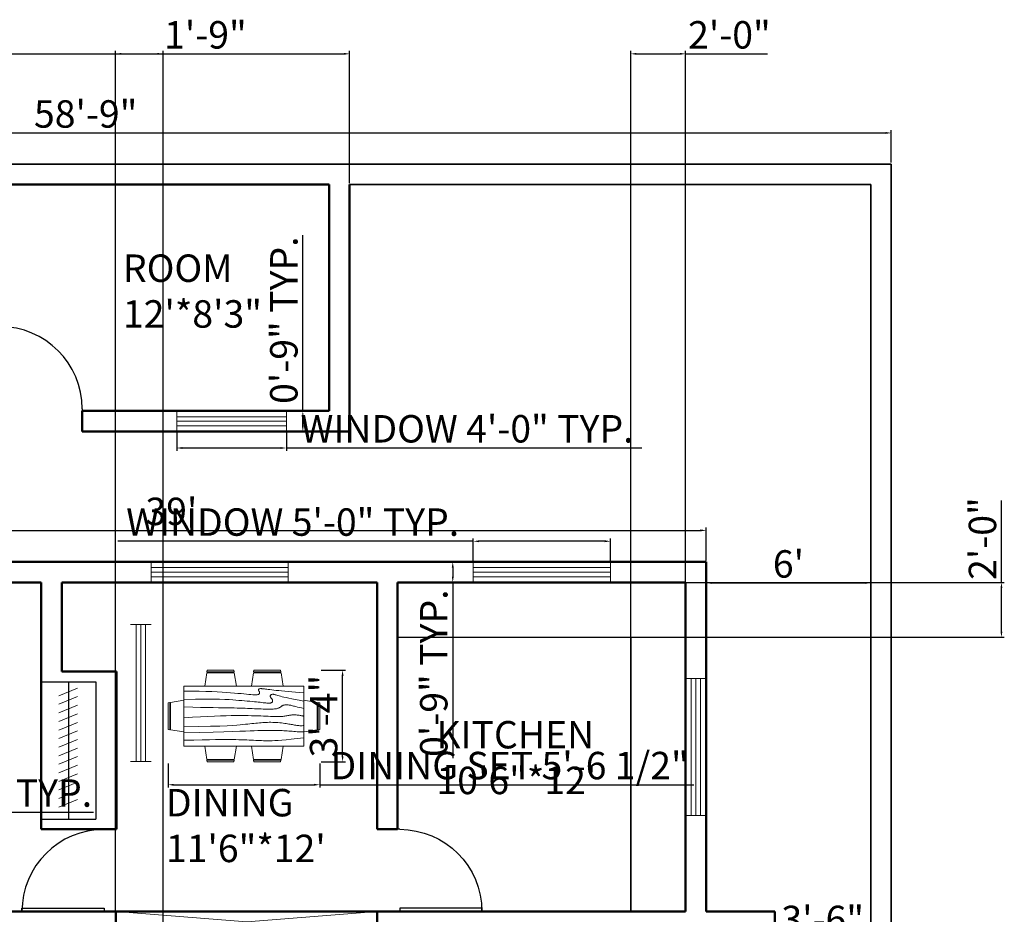
# Model space of a CAD drawing. Units: inches. Extents: x 6286 to 7213, y 5725 to 6776.
# Tile 5 of 5: x 6683 to 7113, y 6385 to 6776. Entities that reach past the tile are written whole.
import ezdxf

# ---------------------------------------------------------------- set-up
doc = ezdxf.new("R2010")
doc.units = ezdxf.units.IN
for name, color, linetype, lineweight in [('A-ANNO-DIMS', 2, 'Continuous', 18), ('A-AREA-IDEN', 7, 'Continuous', 25), ('A-DOOR', 3, 'Continuous', 25), ('A-FLOR-CASE', 8, 'Continuous', 25), ('A-FLOR-CASE-PATT', 252, 'Continuous', 13), ('A-FURN', 8, 'Continuous', 18), ('A-GLAZ', 4, 'Continuous', 18), ('A-WALL', 7, 'Continuous', 50), ('A-WALL-OPEN', 7, 'Continuous', 18), ('C-PROP', 7, 'Continuous', 35)]:
    doc.layers.add(name, color=color, linetype=linetype, lineweight=lineweight)
doc.styles.get("Standard").update_dxf_attribs({"font": 'arial.ttf'})
doc.dimstyles.new('ISO-25', dxfattribs={"dimtxt": 12, "dimasz": 2.5, "dimexe": 1.25, "dimexo": 0.625, "dimtad": 1, "dimdec": 1, "dimlunit": 4, "dimtxsty": 'Standard', "dimcen": 2.5, "dimadec": 0, "dimazin": 0, "dimtfac": 1, "dimtdec": 1, "dimtmove": 0, "dimatfit": 3, "dimfxl": 1, "dimarcsym": 0})

# ---------------------------------------------------------------- blocks, each defined once
blk = doc.blocks.new('*U2')
for p, q in [((0, 0), (0, -6)), ((40, 0), (40, -6))]:
    blk.add_line(p, q)
blk.add_lwpolyline([(0, 0), (0, 40), (1.75, 40), (1.75, 0)], close=True)
blk.add_arc((0, 0), 40, 0, 90)
blk = doc.blocks.new('*D3')
at = {"layer": 'A-ANNO-DIMS', "color": 0, "lineweight": -2, "transparency": 16777216}
for p, q in [((6358.92, 6713.89), (6358.92, 6728.11)), ((6361.42, 6726.86), (7061.42, 6726.86)), ((7063.92, 6713.89), (7063.92, 6728.11))]:
    blk.add_line(p, q, dxfattribs=at)
at = {"layer": 'A-ANNO-DIMS', "color": 0, "lineweight": 100, "transparency": 16777216}
for points in [[(6361.42, 6727.28), (6361.42, 6726.44), (6358.92, 6726.86)], [(7061.42, 6727.28), (7061.42, 6726.44), (7063.92, 6726.86)]]:
    blk.add_solid(points, dxfattribs=at)
at = {"layer": 'Defpoints', "color": 0, "lineweight": 100, "transparency": 16777216}
for p in [(7063.92, 6726.86), (6358.92, 6713.26), (7063.92, 6713.26)]:
    blk.add_point(p, dxfattribs=at)
at = {"layer": 'A-ANNO-DIMS', "color": 0, "transparency": 16777216, "insert": (6711.42, 6733.61), "char_height": 12, "attachment_point": 5}
blk.add_mtext('58\'-9"', dxfattribs=at)
blk = doc.blocks.new('*D5')
at = {"layer": 'A-ANNO-DIMS', "color": 0, "lineweight": -2, "transparency": 16777216}
for p, q in [((6514.92, 6539.89), (6514.92, 6554.27)), ((6517.42, 6553.02), (6980.42, 6553.02)), ((6982.92, 6539.89), (6982.92, 6554.27))]:
    blk.add_line(p, q, dxfattribs=at)
at = {"layer": 'A-ANNO-DIMS', "color": 0, "lineweight": 100, "transparency": 16777216}
for points in [[(6517.42, 6553.44), (6517.42, 6552.6), (6514.92, 6553.02)], [(6980.42, 6553.44), (6980.42, 6552.6), (6982.92, 6553.02)]]:
    blk.add_solid(points, dxfattribs=at)
at = {"layer": 'Defpoints', "color": 0, "lineweight": 100, "transparency": 16777216}
for p in [(6982.92, 6553.02), (6514.92, 6539.26), (6982.92, 6539.26)]:
    blk.add_point(p, dxfattribs=at)
at = {"layer": 'A-ANNO-DIMS', "color": 0, "transparency": 16777216, "insert": (6748.92, 6559.78), "char_height": 12, "attachment_point": 5}
blk.add_mtext("39'", dxfattribs=at)
blk = doc.blocks.new('Dining Set - 36 x 72 in.')
for p, q in [((-22.2343, 26.00059), (-23.4847, 17.99762)), ((-22.2304, 26), (-5.7608, 26)), ((-22, 27.5), (-22.1562, 26.50042)), ((-5.8416, 26.5), (-22.1534, 26.5)), ((-22, 27.5), (-6, 27.5)), ((-5.8437, 26.49966), (-6, 27.5)), ((-4.5152, 17.99762), (-5.7655, 25.99926)), ((5.7657, 26.00059), (4.5153, 17.99762)), ((5.7696, 26), (22.2392, 26)), ((6, 27.5), (5.8438, 26.50042)), ((22.1584, 26.5), (5.8466, 26.5)), ((6, 27.5), (22, 27.5)), ((22.1563, 26.49966), (22, 27.5)), ((23.4848, 17.99762), (22.2345, 25.99926)), ((36, 18), (-36, 18)), ((-36, 18), (-36, -18)), ((36, -18), (36, 18)), ((-45.5, 8), (-44.5004, 8.15617)), ((-45.5, 8), (-45.5, -8)), ((-44.5, -8.15843), (-44.5, 8.15338)), ((-44.0006, 8.23428), (-35.9976, 9.48474)), ((-44, 8.23041), (-44, -8.23915)), ((44.0006, 8.23428), (35.9976, 9.48474)), ((44, 8.23041), (44, -8.23915)), ((44.5, -8.15843), (44.5, 8.15338)), ((45.5, 8), (44.5005, 8.15617)), ((45.5, 8), (45.5, -8)), ((-44.4997, -8.15631), (-45.5, -8)), ((-35.9976, -9.48476), (-43.9993, -8.2345)), ((35.9976, -9.48476), (43.9993, -8.2345)), ((44.4997, -8.15631), (45.5, -8)), ((-36, -18), (36, -18)), ((-22.2343, -26.0006), (-23.4847, -17.99762)), ((-4.5152, -17.99762), (-5.7655, -25.99928)), ((5.7657, -26.0006), (4.5153, -17.99762)), ((23.4848, -17.99762), (22.2345, -25.99928)), ((-22.2304, -26), (-5.7608, -26)), ((-22, -27.5), (-22.1562, -26.50044)), ((-5.8416, -26.5), (-22.1534, -26.5)), ((-22, -27.5), (-6, -27.5)), ((-5.8437, -26.49967), (-6, -27.5)), ((5.7696, -26), (22.2392, -26)), ((6, -27.5), (5.8438, -26.50044)), ((22.1584, -26.5), (5.8466, -26.5)), ((6, -27.5), (22, -27.5)), ((22.1563, -26.49967), (22, -27.5))]:
    blk.add_line(p, q)
for points in [[(-36, 15), (-31.1772, 14.97754), (-26.8079, 14.91406), (-22.8538, 14.81543), (-19.276, 14.6875), (-16.0362, 14.53613), (-13.0957, 14.36718), (-10.4159, 14.18652), (-7.9583, 14), (-5.6904, 13.81315), (-3.6035, 13.63021), (-1.6954, 13.45508), (0.0365, 13.29166), (1.5945, 13.14388), (2.9811, 13.01562), (4.1988, 12.9108), (5.25, 12.83333), (6.1393, 12.78613), (6.8802, 12.76823), (7.4883, 12.77767), (7.9792, 12.8125), (8.3685, 12.87077), (8.6719, 12.95052), (8.9049, 13.0498), (9.0833, 13.16666), (9.2205, 13.29899), (9.3216, 13.44401), (9.3895, 13.59879), (9.4271, 13.76041), (9.4373, 13.92594), (9.4232, 14.09245), (9.3875, 14.257), (9.3333, 14.41666), (9.2638, 14.56917), (9.1836, 14.71484), (9.0975, 14.85465), (9.0104, 14.98958), (8.9272, 15.1206), (8.8529, 15.2487), (8.7922, 15.37483), (8.75, 15.5), (8.7305, 15.62467), (8.7344, 15.74739), (8.7617, 15.86621), (8.8125, 15.97916), (8.8867, 16.08431), (8.9844, 16.17968), (9.1055, 16.26334), (9.25, 16.33333), (9.4189, 16.38802), (9.6172, 16.42708), (9.8506, 16.45052), (10.125, 16.45833), (10.4463, 16.45052), (10.8203, 16.42708), (11.2529, 16.38802), (11.75, 16.33333), (12.3184, 16.26318), (12.9694, 16.17838), (13.7151, 16.07991), (14.5677, 15.96875), (15.5395, 15.84586), (16.6426, 15.71224), (17.8893, 15.56884), (19.2917, 15.41666), (20.859, 15.25667), (22.5879, 15.08984), (24.4721, 14.91715), (26.5052, 14.73958), (28.6809, 14.5581), (30.9929, 14.3737), (33.4347, 14.18733), (36, 14)], [(-36, 10), (-28.9766, 10.14274), (-23.1725, 10.20442), (-18.4241, 10.19775), (-14.5677, 10.13541), (-11.4399, 10.03011), (-8.877, 9.89453), (-6.7154, 9.74137), (-4.7917, 9.58333), (-2.9698, 9.43082), (-1.2246, 9.28515), (0.4415, 9.14534), (2.026, 9.01041), (3.5266, 8.87939), (4.9408, 8.7513), (6.266, 8.62516), (7.5, 8.5), (8.6411, 8.37549), (9.6914, 8.2539), (10.6538, 8.13818), (11.5312, 8.03125), (12.3267, 7.93603), (13.043, 7.85547), (13.6831, 7.79248), (14.25, 7.75), (14.7471, 7.7303), (15.1797, 7.73307), (15.5537, 7.75732), (15.875, 7.80208), (16.1494, 7.86637), (16.3828, 7.94922), (16.5811, 8.04964), (16.75, 8.16666), (16.8944, 8.29915), (17.0143, 8.44531), (17.1089, 8.60319), (17.1771, 8.77083), (17.218, 8.94629), (17.2305, 9.1276), (17.2137, 9.31282), (17.1667, 9.5), (17.0895, 9.6875), (16.987, 9.875), (16.8649, 10.0625), (16.7292, 10.25), (16.5856, 10.4375), (16.4401, 10.625), (16.2985, 10.8125), (16.1667, 11), (16.05, 11.18733), (15.9518, 11.3737), (15.8752, 11.5581), (15.8229, 11.73958), (15.798, 11.91715), (15.8034, 12.08984), (15.842, 12.25667), (15.9167, 12.41666), (16.0295, 12.56836), (16.1784, 12.70833), (16.3605, 12.83268), (16.5729, 12.9375), (16.8127, 13.01888), (17.0768, 13.07291), (17.3625, 13.0957), (17.6667, 13.08333), (17.9894, 13.03312), (18.3418, 12.94726), (18.7382, 12.82918), (19.1927, 12.68229), (19.7195, 12.51001), (20.3327, 12.31575), (21.0465, 12.10294), (21.875, 11.875), (22.8357, 11.63354), (23.959, 11.37304), (25.2786, 11.08618), (26.8282, 10.76562), (28.6414, 10.40405), (30.752, 9.99414), (33.1936, 9.52856), (36, 9)], [(-36, 5.5), (-30.7157, 5.3348), (-26.069, 5.20963), (-21.9946, 5.11767), (-18.4271, 5.05208), (-15.3009, 5.00602), (-12.5508, 4.97265), (-10.1112, 4.94515), (-7.9167, 4.91666), (-5.909, 4.88167), (-4.0586, 4.83984), (-2.3429, 4.79215), (-0.7396, 4.73958), (0.7739, 4.6831), (2.22, 4.6237), (3.6213, 4.56233), (5, 4.5), (6.373, 4.43782), (7.7344, 4.3776), (9.0723, 4.32129), (10.375, 4.27083), (11.6309, 4.22819), (12.8281, 4.19531), (13.9551, 4.17415), (15, 4.16666), (15.954, 4.17448), (16.819, 4.19791), (17.6001, 4.23698), (18.3021, 4.29166), (18.9299, 4.36198), (19.4883, 4.44791), (19.9823, 4.54948), (20.4167, 4.66666), (20.7969, 4.79899), (21.1302, 4.94401), (21.4245, 5.09879), (21.6875, 5.26041), (21.9271, 5.42594), (22.1511, 5.59245), (22.3672, 5.757), (22.5834, 5.91666), (22.8065, 6.06868), (23.0404, 6.21093), (23.2879, 6.34147), (23.5521, 6.45833), (23.8358, 6.55957), (24.142, 6.64323), (24.4735, 6.70735), (24.8334, 6.75), (25.2235, 6.76969), (25.642, 6.76692), (26.0858, 6.74267), (26.5521, 6.69791), (27.0379, 6.63362), (27.5404, 6.55078), (28.0565, 6.45036), (28.5834, 6.33333), (29.1242, 6.19987), (29.7071, 6.04687), (30.3661, 5.87044), (31.1354, 5.66666), (32.0493, 5.43164), (33.142, 5.16146), (34.4475, 4.85221), (36, 4.5)], [(-36, -1), (-30.7915, -0.6591), (-26.0195, -0.38216), (-21.6519, -0.16284), (-17.6563, 0.00521), (-14.0005, 0.12833), (-10.6523, 0.21289), (-7.5796, 0.26522), (-4.75, 0.29166), (-2.134, 0.29793), (0.2878, 0.28711), (2.5317, 0.26163), (4.6146, 0.22396), (6.5529, 0.17651), (8.3633, 0.12174), (10.0623, 0.06209), (11.6667, 0), (13.1899, -0.06201), (14.6341, -0.1211), (15.9982, -0.17432), (17.2813, -0.21875), (18.4823, -0.25147), (19.6003, -0.26953), (20.6343, -0.27002), (21.5834, -0.25), (22.4481, -0.20768), (23.2357, -0.14584), (23.9549, -0.06836), (24.6146, 0.02083), (25.2235, 0.11784), (25.7904, 0.21875), (26.3241, 0.31966), (26.8334, 0.41666), (27.3265, 0.50618), (27.8099, 0.58593), (28.2894, 0.65397), (28.7709, 0.70833), (29.2601, 0.74707), (29.763, 0.76823), (30.2855, 0.76985), (30.8334, 0.75), (31.4088, 0.70784), (31.9994, 0.64713), (32.589, 0.57275), (33.1615, 0.48958), (33.7008, 0.4025), (34.1908, 0.3164), (34.6153, 0.23616), (34.9584, 0.16666), (35.2099, 0.11165), (35.3848, 0.07031), (35.504, 0.04069), (35.5886, 0.02083), (35.6594, 0.00879), (35.7377, 0.0026), (35.8442, 0.00032), (36, 0)], [(-36, -6.5), (-27.1843, -6.31267), (-20.084, -6.1263), (-14.469, -5.9419), (-10.1094, -5.76042), (-6.7752, -5.58285), (-4.2363, -5.41016), (-2.2629, -5.24333), (-0.625, -5.08334), (0.8708, -4.93099), (2.2715, -4.78646), (3.5872, -4.64974), (4.8281, -4.52084), (6.0046, -4.39974), (7.127, -4.28646), (8.2053, -4.18099), (9.25, -4.08334), (10.2705, -3.99382), (11.2734, -3.91407), (12.2647, -3.84603), (13.25, -3.79167), (14.2354, -3.75293), (15.2266, -3.73177), (16.2295, -3.73015), (17.25, -3.75), (18.2912, -3.79248), (19.3451, -3.85547), (20.4009, -3.93604), (21.4479, -4.03125), (22.4754, -4.13819), (23.4727, -4.25391), (24.4289, -4.37549), (25.3334, -4.5), (26.1785, -4.62492), (26.9694, -4.74935), (27.7145, -4.87281), (28.4219, -4.99479), (29.1, -5.11483), (29.7572, -5.23242), (30.4016, -5.34709), (31.0417, -5.45834), (31.6837, -5.56437), (32.3262, -5.65821), (32.9658, -5.73153), (33.599, -5.77604), (34.2224, -5.78345), (34.8327, -5.74545), (35.4264, -5.65373), (36, -5.5)], [(-36, -10), (-26.4022, -9.81299), (-18.4675, -9.62891), (-11.9839, -9.45069), (-6.7396, -9.28125), (-2.5226, -9.12354), (0.8789, -8.98047), (3.6769, -8.85498), (6.0833, -8.75), (8.2767, -8.66765), (10.3021, -8.60677), (12.1712, -8.56543), (13.8958, -8.54167), (15.4876, -8.53353), (16.9583, -8.53907), (18.3197, -8.55632), (19.5834, -8.58334), (20.7616, -8.61841), (21.8685, -8.66081), (22.9188, -8.71004), (23.9271, -8.76563), (24.9081, -8.82707), (25.8763, -8.89388), (26.8465, -8.96558), (27.8334, -9.04167), (28.8474, -9.12118), (29.8828, -9.20117), (30.93, -9.27824), (31.9792, -9.34896), (33.0205, -9.40991), (34.0443, -9.45768), (35.0407, -9.48885), (36, -9.5)], [(-36, -14.5), (-30.0881, -14.33513), (-25.0332, -14.21224), (-20.7312, -14.12647), (-17.0781, -14.07292), (-13.97, -14.04671), (-11.3027, -14.04297), (-8.9724, -14.05681), (-6.875, -14.08334), (-4.9224, -14.11833), (-3.0905, -14.16016), (-1.3709, -14.20785), (0.2448, -14.26042), (1.7647, -14.3169), (3.1973, -14.3763), (4.5507, -14.43767), (5.8333, -14.5), (7.0554, -14.5621), (8.235, -14.62175), (9.3922, -14.67652), (10.5469, -14.72396), (11.7192, -14.76164), (12.929, -14.78711), (14.1965, -14.79794), (15.5417, -14.79167), (16.9933, -14.76424), (18.6152, -14.70508), (20.4804, -14.60197), (22.6615, -14.44271), (25.2312, -14.21509), (28.2624, -13.9069), (31.8277, -13.50594), (36, -13)]]:
    blk.add_lwpolyline(points)
blk = doc.blocks.new('*D23')
at = {"layer": 'A-ANNO-DIMS', "color": 0, "lineweight": -2, "transparency": 16777216}
for p, q in [((6982.92, 6538.64), (6982.92, 6528.79)), ((7054.92, 6538.64), (7054.92, 6528.79)), ((6985.42, 6530.04), (7052.42, 6530.04))]:
    blk.add_line(p, q, dxfattribs=at)
at = {"layer": 'A-ANNO-DIMS', "color": 0, "lineweight": 100, "transparency": 16777216}
for points in [[(6985.42, 6530.45), (6985.42, 6529.62), (6982.92, 6530.04)], [(7052.42, 6530.45), (7052.42, 6529.62), (7054.92, 6530.04)]]:
    blk.add_solid(points, dxfattribs=at)
at = {"layer": 'Defpoints', "color": 0, "lineweight": 100, "transparency": 16777216}
for p in [(6982.92, 6539.26), (7054.92, 6539.26), (7054.92, 6530.04)]:
    blk.add_point(p, dxfattribs=at)
at = {"layer": 'A-ANNO-DIMS', "color": 0, "transparency": 16777216, "insert": (7018.92, 6536.79), "char_height": 12, "attachment_point": 5}
blk.add_mtext("6'", dxfattribs=at)
blk = doc.blocks.new('*D24')
at = {"layer": 'A-ANNO-DIMS', "color": 0, "lineweight": -2, "transparency": 16777216}
for p, q in [((7012.92, 6385.64), (7012.92, 6373.28)), ((7054.92, 6385.64), (7054.92, 6373.28)), ((7015.42, 6374.53), (7052.42, 6374.53))]:
    blk.add_line(p, q, dxfattribs=at)
at = {"layer": 'A-ANNO-DIMS', "color": 0, "lineweight": 100, "transparency": 16777216}
for points in [[(7015.42, 6374.95), (7015.42, 6374.12), (7012.92, 6374.53)], [(7052.42, 6374.95), (7052.42, 6374.12), (7054.92, 6374.53)]]:
    blk.add_solid(points, dxfattribs=at)
at = {"layer": 'Defpoints', "color": 0, "lineweight": 100, "transparency": 16777216}
for p in [(7012.92, 6386.26), (7054.92, 6386.26), (7054.92, 6374.53)]:
    blk.add_point(p, dxfattribs=at)
at = {"layer": 'A-ANNO-DIMS', "color": 0, "transparency": 16777216, "insert": (7033.92, 6381.29), "char_height": 12, "attachment_point": 5}
blk.add_mtext('3\'-6"', dxfattribs=at)
blk = doc.blocks.new('WIN-48IN')
for p, q in [((0, 9), (0, 0)), ((48, 0), (48, 9)), ((0, 6.5), (48, 6.5)), ((0, 4.5), (48, 4.5)), ((0, 2.5), (48, 2.5))]:
    blk.add_line(p, q)
blk = doc.blocks.new('WIN-60IN')
for p, q in [((0, 9), (0, 0)), ((60, 0), (60, 9)), ((60, 6.5), (0, 6.5)), ((60, 4.5), (0, 4.5)), ((60, 2.5), (0, 2.5))]:
    blk.add_line(p, q)
blk = doc.blocks.new('*D35')
at = {"layer": 'A-ANNO-DIMS', "color": 0, "lineweight": -2, "transparency": 16777216}
for p, q in [((6881.04, 6539.89), (6881.04, 6549.51)), ((6941.04, 6539.89), (6941.04, 6549.51)), ((6881.04, 6548.26), (6725.44, 6548.26)), ((6938.54, 6548.26), (6883.54, 6548.26))]:
    blk.add_line(p, q, dxfattribs=at)
at = {"layer": 'A-ANNO-DIMS', "color": 0, "lineweight": 100, "transparency": 16777216}
for points in [[(6883.54, 6548.68), (6883.54, 6547.85), (6881.04, 6548.26)], [(6938.54, 6548.68), (6938.54, 6547.85), (6941.04, 6548.26)]]:
    blk.add_solid(points, dxfattribs=at)
at = {"layer": 'Defpoints', "color": 0, "lineweight": 100, "transparency": 16777216}
for p in [(6881.04, 6548.26), (6881.04, 6539.26), (6941.04, 6539.26)]:
    blk.add_point(p, dxfattribs=at)
at = {"layer": 'A-ANNO-DIMS', "color": 0, "transparency": 16777216, "insert": (6801.99, 6555.1), "char_height": 12, "attachment_point": 5}
blk.add_mtext('WINDOW 5\'-0" TYP.', dxfattribs=at)
blk = doc.blocks.new('*D36')
at = {"layer": 'A-ANNO-DIMS', "color": 0, "lineweight": -2, "transparency": 16777216}
for p, q in [((6880.42, 6539.26), (6870.79, 6539.26)), ((6872.04, 6536.76), (6872.04, 6532.76)), ((6880.42, 6530.26), (6870.79, 6530.26)), ((6872.04, 6530.26), (6872.04, 6453.37))]:
    blk.add_line(p, q, dxfattribs=at)
at = {"layer": 'A-ANNO-DIMS', "color": 0, "lineweight": 100, "transparency": 16777216}
for points in [[(6871.63, 6536.76), (6872.46, 6536.76), (6872.04, 6539.26)], [(6871.63, 6532.76), (6872.46, 6532.76), (6872.04, 6530.26)]]:
    blk.add_solid(points, dxfattribs=at)
at = {"layer": 'Defpoints', "color": 0, "lineweight": 100, "transparency": 16777216}
for p in [(6881.04, 6539.26), (6872.04, 6530.26), (6881.04, 6530.26)]:
    blk.add_point(p, dxfattribs=at)
at = {"layer": 'A-ANNO-DIMS', "color": 0, "transparency": 16777216, "insert": (6865.29, 6490.57), "char_height": 12, "attachment_point": 5, "rotation": 90}
blk.add_mtext('0\'-9" TYP.', dxfattribs=at)
blk = doc.blocks.new('*D37')
at = {"layer": 'A-ANNO-DIMS', "color": 0, "lineweight": -2, "transparency": 16777216}
for p, q in [((6751.24, 6595.64), (6751.24, 6587.81)), ((6799.24, 6595.64), (6799.24, 6587.81)), ((6753.74, 6589.06), (6796.74, 6589.06)), ((6799.24, 6589.06), (6954.84, 6589.06))]:
    blk.add_line(p, q, dxfattribs=at)
at = {"layer": 'A-ANNO-DIMS', "color": 0, "lineweight": 100, "transparency": 16777216}
for points in [[(6753.74, 6589.48), (6753.74, 6588.65), (6751.24, 6589.06)], [(6796.74, 6589.48), (6796.74, 6588.65), (6799.24, 6589.06)]]:
    blk.add_solid(points, dxfattribs=at)
at = {"layer": 'Defpoints', "color": 0, "lineweight": 100, "transparency": 16777216}
for p in [(6751.24, 6596.26), (6799.24, 6596.26), (6799.24, 6589.06)]:
    blk.add_point(p, dxfattribs=at)
at = {"layer": 'A-ANNO-DIMS', "color": 0, "transparency": 16777216, "insert": (6878.29, 6595.9), "char_height": 12, "attachment_point": 5}
blk.add_mtext('WINDOW 4\'-0" TYP.', dxfattribs=at)
blk = doc.blocks.new('*D38')
at = {"layer": 'A-ANNO-DIMS', "color": 0, "lineweight": -2, "transparency": 16777216}
for p, q in [((6806.44, 6605.26), (6806.44, 6682.16)), ((6799.86, 6605.26), (6807.69, 6605.26)), ((6806.44, 6598.76), (6806.44, 6602.76)), ((6799.86, 6596.26), (6807.69, 6596.26))]:
    blk.add_line(p, q, dxfattribs=at)
at = {"layer": 'A-ANNO-DIMS', "color": 0, "lineweight": 100, "transparency": 16777216}
for points in [[(6806.02, 6602.76), (6806.85, 6602.76), (6806.44, 6605.26)], [(6806.02, 6598.76), (6806.85, 6598.76), (6806.44, 6596.26)]]:
    blk.add_solid(points, dxfattribs=at)
at = {"layer": 'Defpoints', "color": 0, "lineweight": 100, "transparency": 16777216}
for p in [(6799.24, 6605.26), (6806.44, 6605.26), (6799.24, 6596.26)]:
    blk.add_point(p, dxfattribs=at)
at = {"layer": 'A-ANNO-DIMS', "color": 0, "transparency": 16777216, "insert": (6799.68, 6644.96), "char_height": 12, "attachment_point": 5, "rotation": 90}
blk.add_mtext('0\'-9" TYP.', dxfattribs=at)
blk = doc.blocks.new('*D48')
at = {"layer": 'A-ANNO-DIMS', "color": 0, "lineweight": -2, "transparency": 16777216}
for p, q in [((6577.92, 6442.12), (6577.92, 6428.58)), ((6637.92, 6442.12), (6637.92, 6428.58)), ((6580.42, 6429.83), (6635.42, 6429.83)), ((6637.92, 6429.83), (6714.82, 6429.83))]:
    blk.add_line(p, q, dxfattribs=at)
at = {"layer": 'A-ANNO-DIMS', "color": 0, "lineweight": 100, "transparency": 16777216}
for points in [[(6580.42, 6430.25), (6580.42, 6429.42), (6577.92, 6429.83)], [(6635.42, 6430.25), (6635.42, 6429.42), (6637.92, 6429.83)]]:
    blk.add_solid(points, dxfattribs=at)
at = {"layer": 'Defpoints', "color": 0, "lineweight": 100, "transparency": 16777216}
for p in [(6577.92, 6442.75), (6637.92, 6442.75), (6637.92, 6429.83)]:
    blk.add_point(p, dxfattribs=at)
at = {"layer": 'A-ANNO-DIMS', "color": 0, "transparency": 16777216, "insert": (6677.62, 6436.59), "char_height": 12, "attachment_point": 5}
blk.add_mtext('5\'-0" TYP.', dxfattribs=at)
blk = doc.blocks.new('*D51')
at = {"layer": 'A-ANNO-DIMS', "color": 0, "lineweight": -2, "transparency": 16777216}
for p, q in [((6747.45, 6451.1), (6747.45, 6440.51)), ((6813.87, 6451.1), (6813.87, 6440.51)), ((6749.95, 6441.76), (6811.37, 6441.76)), ((6813.87, 6441.76), (6977.48, 6441.76))]:
    blk.add_line(p, q, dxfattribs=at)
at = {"layer": 'A-ANNO-DIMS', "color": 0, "lineweight": 100, "transparency": 16777216}
for points in [[(6749.95, 6442.17), (6749.95, 6441.34), (6747.45, 6441.76)], [(6811.37, 6442.17), (6811.37, 6441.34), (6813.87, 6441.76)]]:
    blk.add_solid(points, dxfattribs=at)
at = {"layer": 'Defpoints', "color": 0, "lineweight": 100, "transparency": 16777216}
for p in [(6747.45, 6451.72), (6813.87, 6451.72), (6813.87, 6441.76)]:
    blk.add_point(p, dxfattribs=at)
at = {"layer": 'A-ANNO-DIMS', "color": 0, "transparency": 16777216, "insert": (6896.92, 6448.59), "char_height": 12, "attachment_point": 5}
blk.add_mtext('DINING SET 5\'-6 1/2"', dxfattribs=at)
blk = doc.blocks.new('*D52')
at = {"layer": 'A-ANNO-DIMS', "color": 0, "lineweight": -2, "transparency": 16777216}
for p, q in [((6814.5, 6491.87), (6825.08, 6491.87)), ((6823.83, 6454.22), (6823.83, 6489.37)), ((6814.5, 6451.72), (6825.08, 6451.72))]:
    blk.add_line(p, q, dxfattribs=at)
at = {"layer": 'A-ANNO-DIMS', "color": 0, "lineweight": 100, "transparency": 16777216}
for points in [[(6823.42, 6489.37), (6824.25, 6489.37), (6823.83, 6491.87)], [(6823.42, 6454.22), (6824.25, 6454.22), (6823.83, 6451.72)]]:
    blk.add_solid(points, dxfattribs=at)
at = {"layer": 'Defpoints', "color": 0, "lineweight": 100, "transparency": 16777216}
for p in [(6813.87, 6491.87), (6823.83, 6491.87), (6813.87, 6451.72)]:
    blk.add_point(p, dxfattribs=at)
at = {"layer": 'A-ANNO-DIMS', "color": 0, "transparency": 16777216, "insert": (6817.08, 6471.79), "char_height": 12, "attachment_point": 5, "rotation": 90}
blk.add_mtext('3\'-4"', dxfattribs=at)
blk = doc.blocks.new('*D57')
at = {"layer": 'A-ANNO-DIMS', "color": 0, "lineweight": -2, "transparency": 16777216}
for p, q in [((6358.92, 6713.89), (6358.92, 6762.71)), ((6361.42, 6761.46), (6824.42, 6761.46)), ((6826.92, 6704.89), (6826.92, 6762.71))]:
    blk.add_line(p, q, dxfattribs=at)
at = {"layer": 'A-ANNO-DIMS', "color": 0, "lineweight": 100, "transparency": 16777216}
for points in [[(6361.42, 6761.88), (6361.42, 6761.05), (6358.92, 6761.46)], [(6824.42, 6761.88), (6824.42, 6761.05), (6826.92, 6761.46)]]:
    blk.add_solid(points, dxfattribs=at)
at = {"layer": 'Defpoints', "color": 0, "lineweight": 100, "transparency": 16777216}
for p in [(6826.92, 6761.46), (6358.92, 6713.26), (6826.92, 6704.26)]:
    blk.add_point(p, dxfattribs=at)
at = {"layer": 'A-ANNO-DIMS', "color": 0, "transparency": 16777216, "insert": (6592.92, 6768.22), "char_height": 12, "attachment_point": 5}
blk.add_mtext('39\'-0"', dxfattribs=at)
blk = doc.blocks.new('*D64')
at = {"layer": 'A-ANNO-DIMS', "color": 0, "lineweight": -2, "transparency": 16777216}
for p, q in [((6724.5, 6312.3), (6724.5, 6762.71)), ((6727, 6761.46), (6742.8, 6761.46)), ((6745.3, 6312.3), (6745.3, 6762.71)), ((6745.3, 6761.46), (6779.82, 6761.46))]:
    blk.add_line(p, q, dxfattribs=at)
at = {"layer": 'A-ANNO-DIMS', "color": 0, "lineweight": 100, "transparency": 16777216}
for points in [[(6727, 6761.88), (6727, 6761.05), (6724.5, 6761.46)], [(6742.8, 6761.88), (6742.8, 6761.05), (6745.3, 6761.46)]]:
    blk.add_solid(points, dxfattribs=at)
at = {"layer": 'Defpoints', "color": 0, "lineweight": 100, "transparency": 16777216}
for p in [(6745.3, 6761.46), (6724.5, 6311.67), (6745.3, 6311.67)]:
    blk.add_point(p, dxfattribs=at)
at = {"layer": 'A-ANNO-DIMS', "color": 0, "transparency": 16777216, "insert": (6763.81, 6768.22), "char_height": 12, "attachment_point": 5}
blk.add_mtext('1\'-9"', dxfattribs=at)
blk = doc.blocks.new('*D71')
at = {"layer": 'A-ANNO-DIMS', "color": 0, "lineweight": -2, "transparency": 16777216}
for p, q in [((7112.12, 6530.26), (7112.12, 6566.12)), ((6848.55, 6530.26), (7113.37, 6530.26)), ((7112.12, 6508.76), (7112.12, 6527.76)), ((6848.55, 6506.26), (7113.37, 6506.26))]:
    blk.add_line(p, q, dxfattribs=at)
at = {"layer": 'A-ANNO-DIMS', "color": 0, "lineweight": 100, "transparency": 16777216}
for points in [[(7111.71, 6527.76), (7112.54, 6527.76), (7112.12, 6530.26)], [(7111.71, 6508.76), (7112.54, 6508.76), (7112.12, 6506.26)]]:
    blk.add_solid(points, dxfattribs=at)
at = {"layer": 'Defpoints', "color": 0, "lineweight": 100, "transparency": 16777216}
for p in [(6847.92, 6530.26), (7112.12, 6530.26), (6847.92, 6506.26)]:
    blk.add_point(p, dxfattribs=at)
at = {"layer": 'A-ANNO-DIMS', "color": 0, "transparency": 16777216, "insert": (7105.37, 6549.44), "char_height": 12, "attachment_point": 5, "rotation": 90}
blk.add_mtext('2\'-0"', dxfattribs=at)
blk = doc.blocks.new('*D72')
at = {"layer": 'A-ANNO-DIMS', "color": 0, "lineweight": -2, "transparency": 16777216}
for p, q in [((6949.92, 6386.89), (6949.92, 6762.71)), ((6952.42, 6761.46), (6971.42, 6761.46)), ((6973.92, 6386.89), (6973.92, 6762.71)), ((6973.92, 6761.46), (7009.78, 6761.46))]:
    blk.add_line(p, q, dxfattribs=at)
at = {"layer": 'A-ANNO-DIMS', "color": 0, "lineweight": 100, "transparency": 16777216}
for points in [[(6952.42, 6761.88), (6952.42, 6761.05), (6949.92, 6761.46)], [(6971.42, 6761.88), (6971.42, 6761.05), (6973.92, 6761.46)]]:
    blk.add_solid(points, dxfattribs=at)
at = {"layer": 'Defpoints', "color": 0, "lineweight": 100, "transparency": 16777216}
for p in [(6973.92, 6761.46), (6949.92, 6386.26), (6973.92, 6386.26)]:
    blk.add_point(p, dxfattribs=at)
at = {"layer": 'A-ANNO-DIMS', "color": 0, "transparency": 16777216, "insert": (6993.1, 6768.22), "char_height": 12, "attachment_point": 5}
blk.add_mtext('2\'-0"', dxfattribs=at)

msp = doc.modelspace()

# ---------------------------------------------------------------- hatches: boundary and pattern name
at = {"layer": 'A-FLOR-CASE-PATT'}
h = msp.add_hatch(dxfattribs=at)
h.set_pattern_fill('ANSI31', color=256, scale=1.091306, angle=-22.636, style=0)
h.paths.add_polyline_path([(6699.63, 6428.66), (6707.78, 6432.02), (6707.78, 6484.47), (6699.63, 6481.12)])

# ---------------------------------------------------------------- linework, layer by layer
at = {"layer": 'A-FLOR-CASE'}
for p, q in [((6847.92, 6506.26), (6949.92, 6506.26)), ((6949.92, 6506.26), (6949.92, 6386.26)), ((6691.92, 6486.76), (6715.92, 6486.76)), ((6703.92, 6486.76), (6703.92, 6426.76)), ((6715.92, 6486.76), (6715.92, 6426.76)), ((6691.92, 6426.76), (6715.92, 6426.76))]:
    msp.add_line(p, q, dxfattribs=at)
at = {"layer": 'A-WALL'}
for p, q in [((6673.92, 6704.26), (6817.92, 6704.26)), ((6817.92, 6704.26), (6817.92, 6605.26)), ((6826.92, 6704.26), (6826.92, 6596.26)), ((6709.92, 6605.26), (6817.92, 6605.26)), ((6709.92, 6605.26), (6709.92, 6596.26)), ((6709.92, 6596.26), (6826.92, 6596.26)), ((6514.92, 6539.26), (6982.92, 6539.26)), ((6982.92, 6539.26), (6982.92, 6386.26)), ((6523.92, 6530.26), (6691.92, 6530.26)), ((6691.92, 6530.26), (6691.92, 6422.26)), ((6700.92, 6530.26), (6700.92, 6491.26)), ((6700.92, 6530.26), (6838.92, 6530.26)), ((6838.92, 6530.26), (6838.92, 6422.26)), ((6847.92, 6530.26), (6847.92, 6422.26)), ((6847.92, 6530.26), (6973.92, 6530.26)), ((6973.92, 6530.26), (6973.92, 6386.26)), ((6700.92, 6491.26), (6724.92, 6491.26)), ((6724.92, 6491.26), (6724.92, 6422.26)), ((6691.92, 6422.26), (6724.92, 6422.26)), ((6838.92, 6422.26), (6847.92, 6422.26)), ((6838.92, 6386.26), (6523.92, 6386.26)), ((6838.92, 6386.26), (6838.92, 6117.76)), ((6838.92, 6386.26), (6847.92, 6386.26)), ((6847.92, 6386.26), (6973.92, 6386.26)), ((6982.92, 6386.26), (7012.92, 6386.26)), ((7012.92, 6386.26), (7012.92, 6230.26))]:
    msp.add_line(p, q, dxfattribs=at)
at = {"layer": 'A-WALL-OPEN'}
for p, q in [((6724.92, 6386.26), (6724.92, 6377.26)), ((6724.92, 6386.26), (6838.92, 6377.26)), ((6838.92, 6386.26), (6724.92, 6377.26))]:
    msp.add_line(p, q, dxfattribs=at)
at = {"layer": 'C-PROP'}
for p, q in [((6358.92, 6713.26), (7063.92, 6713.26)), ((7063.92, 6713.26), (7063.92, 5784.76)), ((6826.92, 6704.26), (7054.92, 6704.26)), ((7054.92, 6704.26), (7054.92, 5793.76))]:
    msp.add_line(p, q, dxfattribs=at)

# ---------------------------------------------------------------- block references
at = {"layer": 'A-DOOR', "xscale": 0.9, "yscale": 0.9, "zscale": 0.9}
msp.add_blockref('*U2', (6673.92, 6606.16), dxfattribs=at)
at = {"layer": 'A-DOOR', "yscale": 0.9, "zscale": 0.9}
for p, xscale, rotation in [((6719.52, 6386.26), 0.9, 90.00000000000003), ((6848.82, 6386.26), -0.9, 270)]:
    msp.add_blockref('*U2', p, dxfattribs=dict(at, xscale=xscale, rotation=rotation))
at = {"layer": 'A-FURN', "xscale": 0.7299311223701621, "yscale": 0.7299311223701621, "zscale": 0.7299311223701621}
msp.add_blockref('Dining Set - 36 x 72 in.', (6780.66, 6471.79), dxfattribs=at)
at = {"layer": 'A-GLAZ'}
for name, p in [('WIN-48IN', (6751.24, 6596.26)), ('WIN-60IN', (6740.04, 6530.26))]:
    msp.add_blockref(name, p, dxfattribs=at)
for p, rotation in [((6941.04, 6539.26), 180), ((6740.04, 6451.89), 89.99999999999856), ((6982.92, 6428.26), 90.00000000000026)]:
    msp.add_blockref('WIN-60IN', p, dxfattribs=dict(at, rotation=rotation))

# ---------------------------------------------------------------- texts
at = {"layer": 'A-AREA-IDEN', "char_height": 12, "attachment_point": 1}
for s, width, insert in [('ROOM\\P12\'*8\'3"', 50.4215, (6727.72, 6673.7)), ('KITCHEN\\P10\'6"*12\'', 43.0953, (6864.9, 6469.65)), ('DINING\\P11\'6"*12\'', 54.2585, (6746.53, 6439.92))]:
    msp.add_mtext_dynamic_manual_height_columns(s, width=width, gutter_width=12.5, heights=[0], dxfattribs=dict(at, insert=insert))

# ---------------------------------------------------------------- dimensions: what is measured, and where the dimension line sits
at = {"layer": 'A-ANNO-DIMS'}
for base, p1, p2, override, picture, middle in [((6826.92, 6761.46), (6358.92, 6713.26), (6826.92, 6704.26), {"dimdec": 1, "dimlfac": 1, "dimrnd": 0, "dimzin": 1, "dimdsep": 46, "dimlunit": 4, "dimfrac": 2}, '*D57', (6592.92, 6768.22)), ((6745.3, 6761.46), (6724.5, 6311.67), (6745.3, 6311.67), {"dimdec": 1, "dimlfac": 1, "dimrnd": 0, "dimzin": 1, "dimdsep": 46, "dimlunit": 4, "dimfrac": 2}, '*D64', (6763.81, 6768.22)), ((6973.92, 6761.46), (6949.92, 6386.26), (6973.92, 6386.26), {"dimdec": 1, "dimlfac": 1, "dimrnd": 0, "dimzin": 1, "dimdsep": 46, "dimlunit": 4, "dimfrac": 2}, '*D72', (6993.1, 6768.22)), ((7063.92, 6726.86), (6358.92, 6713.26), (7063.92, 6713.26), {"dimclrd": 0, "dimclre": 0, "dimclrt": 0}, '*D3', (6711.42, 6733.61)), ((6982.92, 6553.02), (6514.92, 6539.26), (6982.92, 6539.26), {"dimclrd": 0, "dimclre": 0, "dimclrt": 0}, '*D5', (6748.92, 6559.78)), ((7054.92, 6530.04), (6982.92, 6539.26), (7054.92, 6539.26), {"dimclrd": 0, "dimclre": 0, "dimclrt": 0}, '*D23', (7018.92, 6536.79)), ((7054.92, 6374.53), (7012.92, 6386.26), (7054.92, 6386.26), {"dimclrd": 0, "dimclre": 0, "dimclrt": 0}, '*D24', (7033.92, 6381.29))]:
    dim = msp.add_linear_dim(base=base, p1=p1, p2=p2, dimstyle='ISO-25', override=override, dxfattribs=at)
    dim.commit()
    dim.dimension.update_dxf_attribs({"geometry": picture, "text_midpoint": middle})
for base, p1, p2, angle, text, picture, middle in [((6806.44, 6605.26), (6799.24, 6596.26), (6799.24, 6605.26), 90, '<> TYP.', '*D38', (6799.68, 6644.96)), ((6881.04, 6548.26), (6941.04, 6539.26), (6881.04, 6539.26), 180, 'WINDOW <> TYP.', '*D35', (6801.99, 6555.1)), ((6872.04, 6530.26), (6881.04, 6539.26), (6881.04, 6530.26), 270, '<> TYP.', '*D36', (6865.29, 6490.57))]:
    dim = msp.add_linear_dim(base=base, p1=p1, p2=p2, angle=angle, text=text, dimstyle='ISO-25', override={"dimdec": 1, "dimlfac": 1, "dimrnd": 0, "dimzin": 1, "dimdsep": 46, "dimlunit": 4, "dimfrac": 2}, dxfattribs=at)
    dim.commit()
    dim.dimension.update_dxf_attribs({"geometry": picture, "text_midpoint": middle})
for base, p1, p2, text, picture, middle in [((6799.24, 6589.06), (6751.24, 6596.26), (6799.24, 6596.26), 'WINDOW <> TYP.', '*D37', (6878.29, 6595.9)), ((6813.87, 6441.76), (6747.45, 6451.72), (6813.87, 6451.72), 'DINING SET <>', '*D51', (6896.92, 6448.59)), ((6637.92, 6429.83), (6577.92, 6442.75), (6637.92, 6442.75), '<> TYP.', '*D48', (6677.62, 6436.59))]:
    dim = msp.add_linear_dim(base=base, p1=p1, p2=p2, text=text, dimstyle='ISO-25', override={"dimdec": 1, "dimlfac": 1, "dimrnd": 0, "dimzin": 1, "dimdsep": 46, "dimlunit": 4, "dimfrac": 2}, dxfattribs=at)
    dim.commit()
    dim.dimension.update_dxf_attribs({"geometry": picture, "text_midpoint": middle})
for base, p1, p2, picture, middle in [((7112.12, 6530.26), (6847.92, 6506.26), (6847.92, 6530.26), '*D71', (7105.37, 6549.44)), ((6823.8343, 6491.8673), (6813.8707, 6451.7211), (6813.8707, 6491.8673), '*D52', (6817.0783, 6471.7942))]:
    dim = msp.add_linear_dim(base=base, p1=p1, p2=p2, angle=90, dimstyle='ISO-25', override={"dimdec": 1, "dimlfac": 1, "dimrnd": 0, "dimzin": 1, "dimdsep": 46, "dimlunit": 4, "dimfrac": 2}, dxfattribs=at)
    dim.commit()
    dim.dimension.update_dxf_attribs({"geometry": picture, "text_midpoint": middle})

doc.saveas('drawing.dxf')
